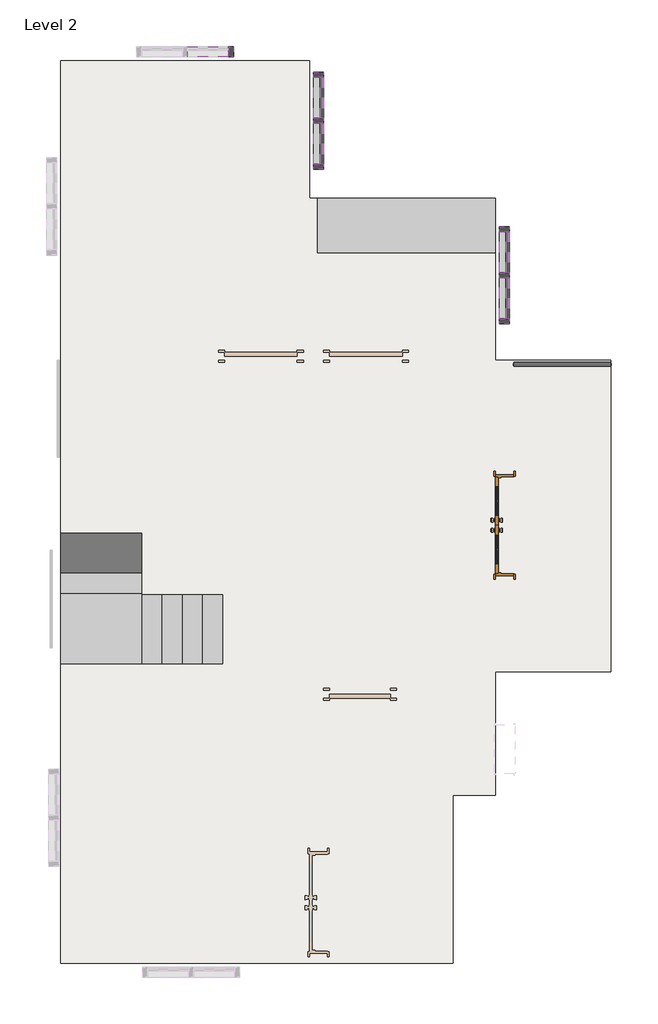
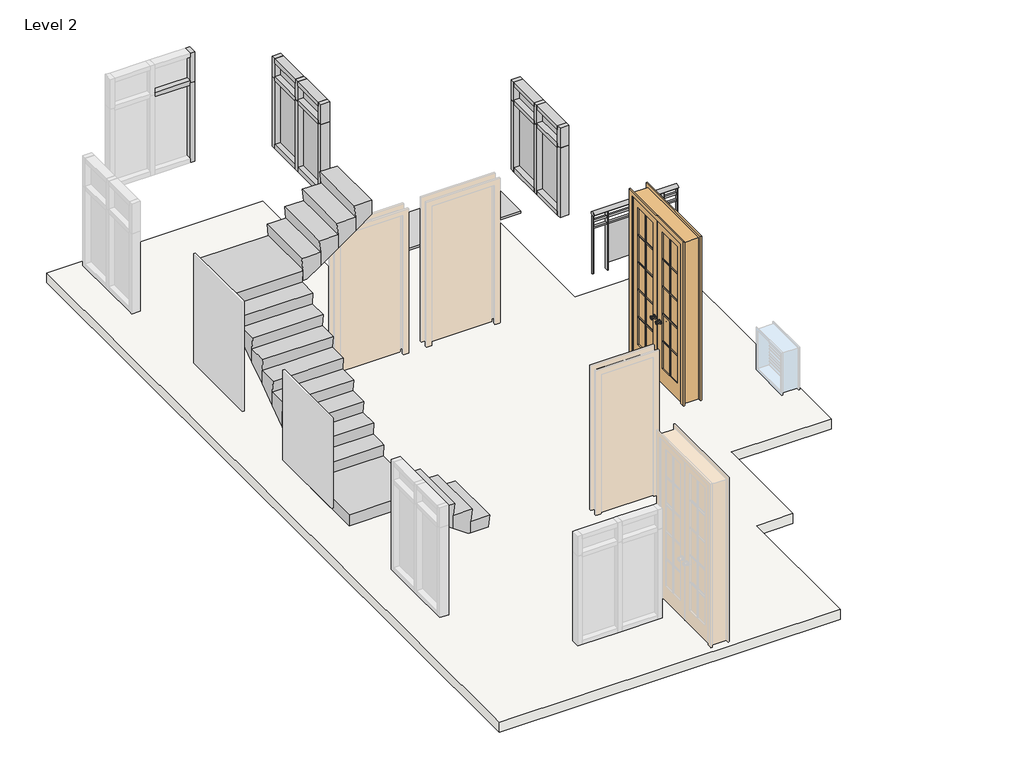
# One storey, part 2 of 2: 27 members, 8 plates, 1 door, 1 furniture element, 1 railing, 1 slab, 1 stair flight.
"""IFC4 building model written with IfcOpenShell, lengths in millimetres."""

from ifc_helpers import new_model, si_unit, point, frame, origin, place, context, project, spatial, polyline, ellipse_curve, trimmed, outline, extrude, faceted_brep, transform, mapped, element, save
from ifc_brep_helpers import plane_surface, extruded_surface, advanced_brep
from components import door_interior_double_full_glass_wood_4_x8_0c92ad92, casework_1_casework_1_edaa4522, member_0b7646a3, member_aaa03826, member_75074519, member_15823cb3, member_75d1e245, member_3c3dc66a, member_a715cb85, member_c4de40ee, system_panel_glazed_63160b6e, system_panel_glazed_4cc38c21

model = new_model("IFC4")

# Units and contexts
model_context = context("Model", 3, world=origin())
ifc_project = project(units=[si_unit("LENGTHUNIT", "METRE", prefix="MILLI")], contexts=[model_context])

# Site, building, storey
site = spatial("IfcSite", under=ifc_project)
building = spatial("IfcBuilding", under=site)
storey = spatial("IfcBuildingStorey", under=building, Name="Level 2", Elevation=609.6)

# Door
placement = place(None, origin())
door_interior_double_full_glass_wood_4_x8_shape = door_interior_double_full_glass_wood_4_x8_0c92ad92(model_context)
element("IfcDoor", 1, ObjectType="Door-Interior-Double-Full Glass-Wood : 4' x8'", at=placement, inside=storey, context=model_context, shape_type="MappedRepresentation", body=[
    mapped(door_interior_double_full_glass_wood_4_x8_shape, transform((738.4084347, 1540.0857557, 609.6), x_axis=(0.0, 1.0, 0.0), y_axis=(-1.0, 0.0, 0.0), z_axis=(0.0, 0.0, 1.0))),
])

# Furniture
casework_1_casework_1_shape = casework_1_casework_1_edaa4522(model_context)
element("IfcFurniture", 2, ObjectType="Casework 1 : Casework 1", at=placement, inside=storey, context=model_context, shape_type="MappedRepresentation", body=[
    mapped(casework_1_casework_1_shape, transform((0.0, 0.0, 0.0), x_axis=(1.0, 0.0, 0.0), y_axis=(0.0, 1.0, 0.0), z_axis=(0.0, 0.0, 1.0))),
])

# Members
member_shape = member_0b7646a3(model_context)
element("IfcMember", 3, ObjectType="Rectangular Mullion : 2.5\" x 5\" rectangular", at=placement, inside=storey, context=model_context, shape_type="MappedRepresentation", body=[
    mapped(member_shape, transform((-1595.2165653, 6068.4899592, 2895.6), x_axis=(0.0, 0.0, 1.0), y_axis=(-1.0, 0.0, 0.0), z_axis=(0.0, -1.0, 0.0))),
])
element("IfcMember", 4, ObjectType="Rectangular Mullion : 2.5\" x 5\" rectangular", at=placement, inside=storey, context=model_context, shape_type="MappedRepresentation", body=[
    mapped(member_shape, transform((-1595.2165653, 6646.3399592, 2895.6), x_axis=(0.0, 0.0, 1.0), y_axis=(-1.0, 0.0, 0.0), z_axis=(0.0, -1.0, 0.0))),
])
element("IfcMember", 5, ObjectType="Rectangular Mullion : 2.5\" x 5\" rectangular", at=placement, inside=storey, context=model_context, shape_type="MappedRepresentation", body=[
    mapped(member_shape, transform((741.5834347, 4130.8857559, 2895.6), x_axis=(0.0, 0.0, 1.0), y_axis=(-1.0, 0.0, 0.0), z_axis=(0.0, -1.0, 0.0))),
])
element("IfcMember", 6, ObjectType="Rectangular Mullion : 2.5\" x 5\" rectangular", at=placement, inside=storey, context=model_context, shape_type="MappedRepresentation", body=[
    mapped(member_shape, transform((741.5834347, 4708.7357559, 2895.6), x_axis=(0.0, 0.0, 1.0), y_axis=(-1.0, 0.0, 0.0), z_axis=(0.0, -1.0, 0.0))),
])
element("IfcMember", 7, ObjectType="Rectangular Mullion : 2.5\" x 5\" rectangular", at=placement, inside=storey, context=model_context, shape_type="MappedRepresentation", body=[
    mapped(member_shape, transform((-1595.2165653, 7160.6899592, 1524.0), x_axis=(0.0, 0.0, -1.0), y_axis=(-1.0, 0.0, 0.0), z_axis=(0.0, 1.0, 0.0))),
])
element("IfcMember", 8, ObjectType="Rectangular Mullion : 2.5\" x 5\" rectangular", at=placement, inside=storey, context=model_context, shape_type="MappedRepresentation", body=[
    mapped(member_shape, transform((-1595.2165653, 6582.8399592, 1524.0), x_axis=(0.0, 0.0, -1.0), y_axis=(-1.0, 0.0, 0.0), z_axis=(0.0, 1.0, 0.0))),
])
element("IfcMember", 9, ObjectType="Rectangular Mullion : 2.5\" x 5\" rectangular", at=placement, inside=storey, context=model_context, shape_type="MappedRepresentation", body=[
    mapped(member_shape, transform((741.5834347, 5223.0857559, 1524.0), x_axis=(0.0, 0.0, -1.0), y_axis=(-1.0, 0.0, 0.0), z_axis=(0.0, 1.0, 0.0))),
])
element("IfcMember", 10, ObjectType="Rectangular Mullion : 2.5\" x 5\" rectangular", at=placement, inside=storey, context=model_context, shape_type="MappedRepresentation", body=[
    mapped(member_shape, transform((741.5834347, 4645.2357559, 1524.0), x_axis=(0.0, 0.0, -1.0), y_axis=(-1.0, 0.0, 0.0), z_axis=(0.0, 1.0, 0.0))),
])
member_2_shape = member_aaa03826(model_context)
element("IfcMember", 11, ObjectType="Rectangular Mullion : 2.5\" x 5\" rectangular", at=placement, inside=storey, context=model_context, shape_type="MappedRepresentation", body=[
    mapped(member_2_shape, transform((-2725.5165655, 7483.6857557, 2743.2), x_axis=(0.0, 0.0, 1.0), y_axis=(0.0, -1.0, 0.0), z_axis=(1.0, 0.0, 0.0))),
])
element("IfcMember", 12, ObjectType="Rectangular Mullion : 2.5\" x 5\" rectangular", at=placement, inside=storey, context=model_context, shape_type="MappedRepresentation", body=[
    mapped(member_2_shape, transform((-1595.2165653, 6646.3399592, 2590.8), x_axis=(0.0, 0.0, 1.0), y_axis=(-1.0, 0.0, 0.0), z_axis=(0.0, -1.0, 0.0))),
])
element("IfcMember", 13, ObjectType="Rectangular Mullion : 2.5\" x 5\" rectangular", at=placement, inside=storey, context=model_context, shape_type="MappedRepresentation", body=[
    mapped(member_2_shape, transform((-1595.2165653, 6068.4899592, 2590.8), x_axis=(0.0, 0.0, 1.0), y_axis=(-1.0, 0.0, 0.0), z_axis=(0.0, -1.0, 0.0))),
])
element("IfcMember", 14, ObjectType="Rectangular Mullion : 2.5\" x 5\" rectangular", at=placement, inside=storey, context=model_context, shape_type="MappedRepresentation", body=[
    mapped(member_2_shape, transform((741.5834347, 4708.7357559, 2590.8), x_axis=(0.0, 0.0, 1.0), y_axis=(-1.0, 0.0, 0.0), z_axis=(0.0, -1.0, 0.0))),
])
element("IfcMember", 15, ObjectType="Rectangular Mullion : 2.5\" x 5\" rectangular", at=placement, inside=storey, context=model_context, shape_type="MappedRepresentation", body=[
    mapped(member_2_shape, transform((741.5834347, 4130.8857559, 2590.8), x_axis=(0.0, 0.0, 1.0), y_axis=(-1.0, 0.0, 0.0), z_axis=(0.0, -1.0, 0.0))),
])
member_3_shape = member_75074519(model_context)
element("IfcMember", 16, ObjectType="Rectangular Mullion : 2.5\" x 5\" rectangular", at=placement, inside=storey, context=model_context, shape_type="MappedRepresentation", body=[
    mapped(member_3_shape, transform((-2662.0165655, 7483.6857557, 1524.0), x_axis=(1.0, 0.0, 0.0), y_axis=(0.0, -1.0, 0.0), z_axis=(0.0, 0.0, -1.0))),
])
member_4_shape = member_15823cb3(model_context)
element("IfcMember", 17, ObjectType="Rectangular Mullion : 2.5\" x 5\" rectangular", at=placement, inside=storey, context=model_context, shape_type="MappedRepresentation", body=[
    mapped(member_4_shape, transform((-2662.0165655, 7483.6857557, 2743.2), x_axis=(1.0, 0.0, 0.0), y_axis=(0.0, -1.0, 0.0), z_axis=(0.0, 0.0, -1.0))),
])
member_5_shape = member_75d1e245(model_context)
element("IfcMember", 18, ObjectType="Rectangular Mullion : 2.5\" x 5\" rectangular", at=placement, inside=storey, context=model_context, shape_type="MappedRepresentation", body=[
    mapped(member_5_shape, transform((-1595.2165653, 6614.5899592, 2590.8), x_axis=(0.0, -1.0, 0.0), y_axis=(-1.0, 0.0, 0.0), z_axis=(0.0, 0.0, -1.0))),
])
element("IfcMember", 19, ObjectType="Rectangular Mullion : 2.5\" x 5\" rectangular", at=placement, inside=storey, context=model_context, shape_type="MappedRepresentation", body=[
    mapped(member_5_shape, transform((741.5834347, 4676.9857559, 2590.8), x_axis=(0.0, -1.0, 0.0), y_axis=(-1.0, 0.0, 0.0), z_axis=(0.0, 0.0, -1.0))),
])
member_6_shape = member_3c3dc66a(model_context)
element("IfcMember", 20, ObjectType="Rectangular Mullion : 2.5\" x 5\" rectangular", at=placement, inside=storey, context=model_context, shape_type="MappedRepresentation", body=[
    mapped(member_6_shape, transform((-1595.2165653, 7224.1899592, 2895.6), x_axis=(0.0, 1.0, 0.0), y_axis=(-1.0, 0.0, 0.0), z_axis=(0.0, 0.0, 1.0))),
])
element("IfcMember", 21, ObjectType="Rectangular Mullion : 2.5\" x 5\" rectangular", at=placement, inside=storey, context=model_context, shape_type="MappedRepresentation", body=[
    mapped(member_6_shape, transform((741.5834347, 5286.5857559, 2895.6), x_axis=(0.0, 1.0, 0.0), y_axis=(-1.0, 0.0, 0.0), z_axis=(0.0, 0.0, 1.0))),
])
element("IfcMember", 22, ObjectType="Rectangular Mullion : 2.5\" x 5\" rectangular", at=placement, inside=storey, context=model_context, shape_type="MappedRepresentation", body=[
    mapped(member_6_shape, transform((-1595.2165653, 6004.9899592, 2590.8), x_axis=(0.0, -1.0, 0.0), y_axis=(-1.0, 0.0, 0.0), z_axis=(0.0, 0.0, -1.0))),
])
element("IfcMember", 23, ObjectType="Rectangular Mullion : 2.5\" x 5\" rectangular", at=placement, inside=storey, context=model_context, shape_type="MappedRepresentation", body=[
    mapped(member_6_shape, transform((741.5834347, 4067.3857559, 2590.8), x_axis=(0.0, -1.0, 0.0), y_axis=(-1.0, 0.0, 0.0), z_axis=(0.0, 0.0, -1.0))),
])
member_7_shape = member_a715cb85(model_context)
element("IfcMember", 24, ObjectType="Rectangular Mullion : 2.5\" x 5\" rectangular", at=placement, inside=storey, context=model_context, shape_type="MappedRepresentation", body=[
    mapped(member_7_shape, transform((-1595.2165653, 6614.5899592, 1524.0), x_axis=(0.0, -1.0, 0.0), y_axis=(-1.0, 0.0, 0.0), z_axis=(0.0, 0.0, -1.0))),
])
element("IfcMember", 25, ObjectType="Rectangular Mullion : 2.5\" x 5\" rectangular", at=placement, inside=storey, context=model_context, shape_type="MappedRepresentation", body=[
    mapped(member_7_shape, transform((741.5834347, 4676.9857559, 1524.0), x_axis=(0.0, -1.0, 0.0), y_axis=(-1.0, 0.0, 0.0), z_axis=(0.0, 0.0, -1.0))),
])
member_8_shape = member_c4de40ee(model_context)
element("IfcMember", 26, ObjectType="Rectangular Mullion : 2.5\" x 5\" rectangular", at=placement, inside=storey, context=model_context, shape_type="MappedRepresentation", body=[
    mapped(member_8_shape, transform((-1595.2165653, 6004.9899592, 1524.0), x_axis=(0.0, -1.0, 0.0), y_axis=(-1.0, 0.0, 0.0), z_axis=(0.0, 0.0, -1.0))),
])
element("IfcMember", 27, ObjectType="Rectangular Mullion : 2.5\" x 5\" rectangular", at=placement, inside=storey, context=model_context, shape_type="MappedRepresentation", body=[
    mapped(member_8_shape, transform((741.5834347, 4067.3857559, 1524.0), x_axis=(0.0, -1.0, 0.0), y_axis=(-1.0, 0.0, 0.0), z_axis=(0.0, 0.0, -1.0))),
])
element("IfcMember", 28, ObjectType="Rectangular Mullion : 2.5\" x 5\" rectangular", at=placement, inside=storey, context=model_context, shape_type="MappedRepresentation", body=[
    mapped(member_8_shape, transform((-1595.2165653, 7224.1899592, 2590.8), x_axis=(0.0, 1.0, 0.0), y_axis=(-1.0, 0.0, 0.0), z_axis=(0.0, 0.0, 1.0))),
])
element("IfcMember", 29, ObjectType="Rectangular Mullion : 2.5\" x 5\" rectangular", at=placement, inside=storey, context=model_context, shape_type="MappedRepresentation", body=[
    mapped(member_8_shape, transform((741.5834347, 5286.5857559, 2590.8), x_axis=(0.0, 1.0, 0.0), y_axis=(-1.0, 0.0, 0.0), z_axis=(0.0, 0.0, 1.0))),
])

# Plates
system_panel_glazed_shape = system_panel_glazed_63160b6e(model_context)
element("IfcPlate", 30, ObjectType="System Panel : Glazed", at=placement, inside=storey, context=model_context, shape_type="MappedRepresentation", body=[
    mapped(system_panel_glazed_shape, transform((741.5834347, 4965.9107559, 2622.55), x_axis=(0.0, -1.0, 0.0), y_axis=(1.0, 0.0, 0.0), z_axis=(0.0, 0.0, 1.0))),
])
element("IfcPlate", 31, ObjectType="System Panel : Glazed", at=placement, inside=storey, context=model_context, shape_type="MappedRepresentation", body=[
    mapped(system_panel_glazed_shape, transform((741.5834347, 4388.0607559, 2622.55), x_axis=(0.0, -1.0, 0.0), y_axis=(1.0, 0.0, 0.0), z_axis=(0.0, 0.0, 1.0))),
])
element("IfcPlate", 32, ObjectType="System Panel : Glazed", at=placement, inside=storey, context=model_context, shape_type="MappedRepresentation", body=[
    mapped(system_panel_glazed_shape, transform((-1595.2165653, 6903.5149592, 2622.55), x_axis=(0.0, -1.0, 0.0), y_axis=(1.0, 0.0, 0.0), z_axis=(0.0, 0.0, 1.0))),
])
element("IfcPlate", 33, ObjectType="System Panel : Glazed", at=placement, inside=storey, context=model_context, shape_type="MappedRepresentation", body=[
    mapped(system_panel_glazed_shape, transform((-1595.2165653, 6325.6649592, 2622.55), x_axis=(0.0, -1.0, 0.0), y_axis=(1.0, 0.0, 0.0), z_axis=(0.0, 0.0, 1.0))),
])
system_panel_glazed_2_shape = system_panel_glazed_4cc38c21(model_context)
element("IfcPlate", 34, ObjectType="System Panel : Glazed", at=placement, inside=storey, context=model_context, shape_type="MappedRepresentation", body=[
    mapped(system_panel_glazed_2_shape, transform((-1595.2165653, 6903.5149592, 1587.5), x_axis=(0.0, -1.0, 0.0), y_axis=(1.0, 0.0, 0.0), z_axis=(0.0, 0.0, 1.0))),
])
element("IfcPlate", 35, ObjectType="System Panel : Glazed", at=placement, inside=storey, context=model_context, shape_type="MappedRepresentation", body=[
    mapped(system_panel_glazed_2_shape, transform((741.5834347, 4965.9107559, 1587.5), x_axis=(0.0, -1.0, 0.0), y_axis=(1.0, 0.0, 0.0), z_axis=(0.0, 0.0, 1.0))),
])
element("IfcPlate", 36, ObjectType="System Panel : Glazed", at=placement, inside=storey, context=model_context, shape_type="MappedRepresentation", body=[
    mapped(system_panel_glazed_2_shape, transform((741.5834347, 4388.0607559, 1587.5), x_axis=(0.0, -1.0, 0.0), y_axis=(1.0, 0.0, 0.0), z_axis=(0.0, 0.0, 1.0))),
])
element("IfcPlate", 37, ObjectType="System Panel : Glazed", at=placement, inside=storey, context=model_context, shape_type="MappedRepresentation", body=[
    mapped(system_panel_glazed_2_shape, transform((-1595.2165653, 6325.6649592, 1587.5), x_axis=(0.0, -1.0, 0.0), y_axis=(1.0, 0.0, 0.0), z_axis=(0.0, 0.0, 1.0))),
])

# Railing
element("IfcRailing", 38, ObjectType="Glass Panel - Bottom Fill", at=placement, inside=storey, context=model_context, shape_type="SolidModel", body=[
    advanced_brep(
    [(855.8834347, 3597.4857557, 1828.8), (855.8834347, 3521.2857557, 1828.8), (2075.0834347, 3597.4857557, 1828.8), (2075.0834347, 3521.2857557, 1828.8)],
    [
        (0, 1, ellipse_curve(frame((855.8834347, 3559.3857557, 1828.8), z_axis=(-1.0, 0.0, 0.0), x_axis=(0.0, -1.0, 0.0)), 38.1, 28.575)),
        (1, 0, ellipse_curve(frame((855.8834347, 3559.3857557, 1828.8), z_axis=(-1.0, 0.0, 0.0), x_axis=(0.0, -1.0, 0.0)), 38.1, 28.575)),
        (2, 3, ellipse_curve(frame((2075.0834347, 3559.3857557, 1828.8), z_axis=(1.0, 0.0, 0.0), x_axis=(0.0, -1.0, 0.0)), 38.1, 28.575)),
        (3, 2, ellipse_curve(frame((2075.0834347, 3559.3857557, 1828.8), z_axis=(1.0, 0.0, 0.0), x_axis=(0.0, -1.0, 0.0)), 38.1, 28.575)),
        (0, 2),
        (3, 1),
    ],
    [
        plane_surface(frame((855.8834347, 3559.3857557, 1828.8), z_axis=(-1.0, 0.0, 0.0), x_axis=(0.0, 1.0, 0.0))),
        plane_surface(frame((2075.0834347, 3559.3857557, 1828.8), z_axis=(1.0, 0.0, 0.0), x_axis=(0.0, 1.0, 0.0))),
        extruded_surface(trimmed(ellipse_curve(frame((2075.0834347, 3559.3857557, 1828.8), z_axis=(-1.0, 0.0, 0.0), x_axis=(0.0, -1.0, 0.0)), 38.1, 28.575), [point((2075.0834347, 3597.4857557, 1828.8))], [point((2075.0834347, 3521.2857557, 1828.8))], True, "CARTESIAN"), (-1219.2, 0.0, 0.0), 1219.2),
        extruded_surface(trimmed(ellipse_curve(frame((2075.0834347, 3559.3857557, 1828.8), z_axis=(-1.0, 0.0, 0.0), x_axis=(0.0, -1.0, 0.0)), 38.1, 28.575), [point((2075.0834347, 3521.2857557, 1828.8))], [point((2075.0834347, 3597.4857557, 1828.8))], True, "CARTESIAN"), (-1219.2, 0.0, 0.0), 1219.2),
    ],
    [
        (0, [[1, 2]]),
        (1, [[3, 4]]),
        (2, [[-1, 5, -4, 6]]),
        (3, [[-2, -6, -3, -5]]),
    ],
),
    extrude(outline(polyline([(855.8834347, 3546.6857557), (855.8834347, 3572.0857557), (2075.0834347, 3572.0857557), (2075.0834347, 3546.6857557), (855.8834347, 3546.6857557)])), frame((0.0, 0.0, 1714.5), z_axis=(0.0, 0.0, 1.0), x_axis=(1.0, 0.0, 0.0)), (0.0, 0.0, 1.0), 25.4),
    extrude(outline(polyline([(855.8834347, 3546.6857557), (855.8834347, 3572.0857557), (2075.0834347, 3572.0857557), (2075.0834347, 3546.6857557), (855.8834347, 3546.6857557)])), frame((0.0, 0.0, 1612.9), z_axis=(0.0, 0.0, 1.0), x_axis=(1.0, 0.0, 0.0)), (0.0, 0.0, 1.0), 25.4),
    extrude(outline(polyline([(1865.5334347, 3533.9857557), (1865.5334347, 3584.7857557), (1878.2334347, 3584.7857557), (1878.2334347, 3533.9857557), (1865.5334347, 3533.9857557)])), frame((0.0, 0.0, 914.4), z_axis=(0.0, 0.0, 1.0), x_axis=(1.0, 0.0, 0.0)), (0.0, 0.0, 1.0), 885.825),
    extrude(outline(polyline([(1059.0834347, 3565.9209127), (1871.8834347, 3565.9209127), (1871.8834347, 3559.5709127), (1059.0834347, 3559.5709127), (1059.0834347, 3565.9209127)])), frame((0.0, 0.0, 1016.0), z_axis=(0.0, 0.0, 1.0), x_axis=(1.0, 0.0, 0.0)), (0.0, 0.0, 1.0), 596.9),
    extrude(outline(polyline([(1052.7334347, 3533.9857557), (1052.7334347, 3584.7857557), (1065.4334347, 3584.7857557), (1065.4334347, 3533.9857557), (1052.7334347, 3533.9857557)])), frame((0.0, 0.0, 914.4), z_axis=(0.0, 0.0, 1.0), x_axis=(1.0, 0.0, 0.0)), (0.0, 0.0, 1.0), 885.825),
    extrude(outline(polyline([(2062.3834347, 3549.8607557), (2062.3834347, 3568.9107557), (2081.4334347, 3568.9107557), (2081.4334347, 3549.8607557), (2062.3834347, 3549.8607557)])), frame((0.0, 0.0, 914.4), z_axis=(0.0, 0.0, 1.0), x_axis=(1.0, 0.0, 0.0)), (0.0, 0.0, 1.0), 885.825),
    extrude(outline(polyline([(849.5334347, 3549.8607557), (849.5334347, 3568.9107557), (868.5834347, 3568.9107557), (868.5834347, 3549.8607557), (849.5334347, 3549.8607557)])), frame((0.0, 0.0, 914.4), z_axis=(0.0, 0.0, 1.0), x_axis=(1.0, 0.0, 0.0)), (0.0, 0.0, 1.0), 885.825),
])

# Slab
element("IfcSlab", 39, ObjectType="6\" floor", at=placement, inside=storey, context=model_context, shape_type="SweptSolid", body=[
    extrude(outline(polyline([(-1709.5165653, 7369.3857557), (-1709.5165653, 5642.1857557), (627.2834347, 5642.1857557), (627.2834347, 3610.1857557), (2075.0834347, 3610.1857557), (2075.0834347, -301.4142443), (627.2834347, -301.4142443), (627.2834347, -1850.8142443), (93.8834347, -1850.8142443), (93.8834347, -3959.0142443), (-4833.7165653, -3959.0142443), (-4833.7165653, 7369.3857557), (-1709.5165653, 7369.3857557)])), frame((0.0, 0.0, 457.2), z_axis=(0.0, 0.0, 1.0), x_axis=(1.0, 0.0, 0.0)), (0.0, 0.0, 1.0), 152.4),
])

# Stair flight
element("IfcStairFlight", 40, ObjectType="3/4\" Nosing 6 1/2\" Depth", at=placement, inside=storey, context=model_context, shape_type="Brep", body=[
    faceted_brep([(-2801.7165653, 663.7857557, 787.4), (-2801.7165653, -199.8142443, 787.4), (-2820.7665653, -199.8142443, 609.6), (-2820.7665653, 663.7857557, 609.6), (-3074.7665653, 663.7857557, 787.4), (-3074.7665653, -199.8142443, 787.4), (-3074.7665653, -199.8142443, 609.6), (-3074.7665653, 663.7857557, 609.6), (-3055.7165653, -199.8142443, 965.2), (-3055.7165653, 663.7857557, 965.2), (-3328.7665653, 663.7857557, 965.2), (-3328.7665653, -199.8142443, 965.2), (-3328.7665653, -199.8142443, 763.6697668), (-3108.6668985, -199.8142443, 609.6), (-3108.6668985, 663.7857557, 609.6), (-3328.7665653, 663.7857557, 763.6697668), (-3309.7165653, -199.8142443, 1143.0), (-3309.7165653, 663.7857557, 1143.0), (-3582.7665653, 663.7857557, 1143.0), (-3582.7665653, -199.8142443, 1143.0), (-3582.7665653, -199.8142443, 941.4697668), (-3582.7665653, 663.7857557, 941.4697668), (-3563.7165653, -199.8142443, 1320.8), (-3563.7165653, 663.7857557, 1320.8), (-3836.7665653, 663.7857557, 1320.8), (-3836.7665653, -199.8142443, 1320.8), (-3836.7665653, -199.8142443, 1119.2697668), (-4142.8097556, 663.7857557, 1333.5), (-3835.405851, 663.7857557, 1333.5), (-4833.7165653, 704.6678432, 1498.6), (-4833.7165653, -199.8142443, 1498.6), (-4142.8097556, -199.8142443, 1498.6), (-3817.7165653, -199.8142443, 1498.6), (-3817.7165653, 663.7857557, 1498.6), (-3817.7165653, 704.6678432, 1498.6), (-4833.7165653, 704.6678432, 1333.5), (-4833.7165653, -199.8142443, 1333.5), (-4142.8097556, -199.8142443, 1333.5), (-3817.7165653, 663.7857557, 1333.5), (-3817.7165653, 704.6678432, 1333.5), (-4833.7165653, 685.6178432, 1676.4), (-3817.7165653, 685.6178432, 1676.4), (-3817.7165653, 756.7110335, 1676.4), (-3817.7165653, 958.6678432, 1676.4), (-4833.7165653, 958.6678432, 1676.4), (-4833.7165653, 756.7110335, 1676.4), (-4833.7165653, 958.6678432, 1474.8697668), (-4833.7165653, 756.7110335, 1333.5), (-3817.7165653, 756.7110335, 1333.5), (-3817.7165653, 958.6678432, 1474.8697668), (-4833.7165653, 939.6178432, 1854.2), (-3817.7165653, 939.6178432, 1854.2), (-3817.7165653, 1212.6678432, 1854.2), (-4833.7165653, 1212.6678432, 1854.2), (-4833.7165653, 1212.6678432, 1652.6697668), (-3817.7165653, 1212.6678432, 1652.6697668), (-4833.7165653, 1193.6178432, 2032.0), (-3817.7165653, 1193.6178432, 2032.0), (-3817.7165653, 1466.6678432, 2032.0), (-4833.7165653, 1466.6678432, 2032.0), (-4833.7165653, 1466.6678432, 1830.4697668), (-3817.7165653, 1466.6678432, 1830.4697668), (-4833.7165653, 1447.6178432, 2209.8), (-3817.7165653, 1447.6178432, 2209.8), (-3817.7165653, 1720.6678432, 2209.8), (-4833.7165653, 1720.6678432, 2209.8), (-4833.7165653, 1720.6678432, 2008.2697668), (-3817.7165653, 1720.6678432, 2008.2697668), (-4833.7165653, 1701.6178432, 2387.6), (-3817.7165653, 1701.6178432, 2387.6), (-3817.7165653, 1974.6678432, 2387.6), (-4833.7165653, 1974.6678432, 2387.6), (-4833.7165653, 1974.6678432, 2186.0697668), (-3817.7165653, 1974.6678432, 2186.0697668), (-4833.7165653, 1955.6178432, 2565.4), (-3817.7165653, 1955.6178432, 2565.4), (-3817.7165653, 2228.6678432, 2565.4), (-4833.7165653, 2228.6678432, 2565.4), (-4833.7165653, 2228.6678432, 2363.8697668), (-3817.7165653, 2228.6678432, 2363.8697668), (-4833.7165653, 2209.6178432, 2743.2), (-3817.7165653, 2209.6178432, 2743.2), (-3817.7165653, 2482.6678432, 2743.2), (-4833.7165653, 2482.6678432, 2743.2), (-4833.7165653, 2482.6678432, 2541.6697668), (-3817.7165653, 2482.6678432, 2541.6697668), (-4833.7165653, 2463.6178432, 2921.0), (-3817.7165653, 2463.6178432, 2921.0), (-3817.7165653, 2736.6678432, 2921.0), (-4833.7165653, 2736.6678432, 2921.0), (-4833.7165653, 2736.6678432, 2719.4697668), (-3817.7165653, 2736.6678432, 2719.4697668), (-3798.6665653, 3610.1857557, 3098.8), (-4833.7165653, 3610.1857557, 3098.8), (-4833.7165653, 3042.7110335, 3098.8), (-4833.7165653, 2717.6178432, 3098.8), (-3817.7165653, 2717.6178432, 3098.8), (-3817.7165653, 2746.5857557, 3098.8), (-3798.6665653, 2746.5857557, 3098.8), (-3798.6665653, 3610.1857557, 2933.7), (-4833.7165653, 3610.1857557, 2933.7), (-4833.7165653, 3042.7110335, 2933.7), (-3817.7165653, 3042.7110335, 2933.7), (-3817.7165653, 2746.5857557, 2933.7), (-3798.6665653, 2746.5857557, 2933.7), (-3817.7165653, 3610.1857557, 3276.6), (-3817.7165653, 2746.5857557, 3276.6), (-3746.623375, 2746.5857557, 3276.6), (-3544.6665653, 2746.5857557, 3276.6), (-3544.6665653, 3610.1857557, 3276.6), (-3746.623375, 3610.1857557, 3276.6), (-3544.6665653, 3610.1857557, 3075.0697668), (-3746.623375, 3610.1857557, 2933.7), (-3746.623375, 2746.5857557, 2933.7), (-3544.6665653, 2746.5857557, 3075.0697668), (-3563.7165653, 3610.1857557, 3454.4), (-3563.7165653, 2746.5857557, 3454.4), (-3290.6665653, 2746.5857557, 3454.4), (-3290.6665653, 3610.1857557, 3454.4), (-3290.6665653, 3610.1857557, 3252.8697668), (-3290.6665653, 2746.5857557, 3252.8697668), (-3309.7165653, 3610.1857557, 3632.2), (-3309.7165653, 2746.5857557, 3632.2), (-3036.6665653, 2746.5857557, 3632.2), (-3036.6665653, 3610.1857557, 3632.2), (-3036.6665653, 3610.1857557, 3430.6697668), (-3036.6665653, 2746.5857557, 3430.6697668), (-3055.7165653, 3610.1857557, 3810.0), (-3055.7165653, 2746.5857557, 3810.0), (-2801.7165653, 2746.5857557, 3810.0), (-2801.7165653, 3610.1857557, 3810.0), (-2801.7165653, 3610.1857557, 3595.1347668), (-2801.7165653, 2746.5857557, 3595.1347668)], [[[0, 1, 2, 3]], [[1, 0, 4, 5]], [[1, 5, 6, 2]], [[4, 0, 3, 7]], [[8, 9, 10, 11]], [[6, 5, 8, 11, 12, 13]], [[4, 7, 14, 15, 10, 9]], [[5, 4, 9, 8]], [[16, 17, 18, 19]], [[16, 19, 20, 12, 11]], [[18, 17, 10, 15, 21]], [[11, 10, 17, 16]], [[22, 23, 24, 25]], [[22, 25, 26, 20, 19]], [[23, 18, 21, 27, 28, 24]], [[19, 18, 23, 22]], [[29, 30, 31, 32, 33, 34]], [[30, 29, 35, 36]], [[25, 32, 31, 30, 36, 37, 26]], [[33, 28, 38]], [[34, 33, 38, 39]], [[25, 24, 28, 33, 32]], [[40, 41, 42, 43, 44, 45]], [[29, 40, 45, 44, 46, 47, 35]], [[41, 34, 39, 48, 49, 43, 42]], [[29, 34, 41, 40]], [[50, 51, 52, 53]], [[50, 53, 54, 46, 44]], [[52, 51, 43, 49, 55]], [[44, 43, 51, 50]], [[56, 57, 58, 59]], [[56, 59, 60, 54, 53]], [[58, 57, 52, 55, 61]], [[53, 52, 57, 56]], [[62, 63, 64, 65]], [[62, 65, 66, 60, 59]], [[64, 63, 58, 61, 67]], [[59, 58, 63, 62]], [[68, 69, 70, 71]], [[68, 71, 72, 66, 65]], [[70, 69, 64, 67, 73]], [[65, 64, 69, 68]], [[74, 75, 76, 77]], [[74, 77, 78, 72, 71]], [[76, 75, 70, 73, 79]], [[71, 70, 75, 74]], [[80, 81, 82, 83]], [[80, 83, 84, 78, 77]], [[82, 81, 76, 79, 85]], [[77, 76, 81, 80]], [[86, 87, 88, 89]], [[86, 89, 90, 84, 83]], [[88, 87, 82, 85, 91]], [[83, 82, 87, 86]], [[92, 93, 94, 95, 96, 97, 98]], [[93, 92, 99, 100]], [[89, 95, 94, 93, 100, 101, 90]], [[97, 96, 88, 91, 102, 103]], [[98, 97, 103, 104]], [[89, 88, 96, 95]], [[105, 106, 107, 108, 109, 110]], [[92, 105, 110, 109, 111, 112, 99]], [[106, 98, 104, 113, 114, 108, 107]], [[92, 98, 106, 105]], [[115, 116, 117, 118]], [[115, 118, 119, 111, 109]], [[117, 116, 108, 114, 120]], [[109, 108, 116, 115]], [[121, 122, 123, 124]], [[121, 124, 125, 119, 118]], [[123, 122, 117, 120, 126]], [[118, 117, 122, 121]], [[127, 128, 129, 130]], [[127, 130, 131, 125, 124]], [[129, 128, 123, 126, 132]], [[130, 129, 132, 131]], [[124, 123, 128, 127]], [[2, 6, 13, 14, 7, 3]], [[37, 27, 21, 15, 14, 13, 12, 20, 26]], [[27, 37, 36, 35, 47, 48, 39, 38, 28]], [[48, 47, 46, 54, 60, 66, 72, 78, 84, 90, 101, 102, 91, 85, 79, 73, 67, 61, 55, 49]], [[102, 101, 100, 99, 112, 113, 104, 103]], [[113, 112, 111, 119, 125, 131, 132, 126, 120, 114]]]),
])

save(model, "model.ifc")

# Revit data of these elements
# Type "Door-Interior-Double-Full Glass-Wood : 4' x8'"
#   Type Mark = "14"
#   Assembly Code = "C1020300"
#   Analytic Construction = "French door, wood frame with single glass"
#   Top Rail = 0' - 4 11/16"
#   Thickness = 0' - 1 3/8"
#   Thermal Resistance (R) = 1.0696 (h·ft²·°F)/BTU
#   Swing Angle [instance default] = 90.00°
#   Stiles = 0' - 4 3/4"
#   Rough Width = 4' - 2"
#   Rough Height = 8' - 1"
#   Panel Width = 2' - 0"
#   Height = 8' - 0"
#   Width = 4' - 0"
#   Heat Transfer Coefficient (U) = 0.9350 BTU/(h·ft²·°F)
#   Bottom Rail = 0' - 9 1/8"
#   Show Grill [instance default] = yes
#   Trim Material = Cherry
#   Panel Material = Cherry
#   Frame Material = Cherry
#   Door Handle Material = Aluminum
#   Visual Light Transmittance = 0
#   Solar Heat Gain Coefficient = 0
#   Wall Closure = (empty or 0)
#   Function = (empty or 0)
# Type "Rectangular Mullion : 2.5\" x 5\" rectangular"
#   built-in parameter 1007304 = 0.416667 (stored number, unit not read)
#   built-in parameter 1007301 = 0.104167 (stored number, unit not read)
#   built-in parameter 1007300 = 0.104167 (stored number, unit not read)
# Type "System Panel : Glazed"
#   Construction Type Id = "GSP4R"
#   Analytic Construction = "1/8 in Pilkington single glazing"
#   Visual Light Transmittance = 0.9
#   Solar Heat Gain Coefficient = 0.86
#   Heat Transfer Coefficient (U) = 1.18115 BTU/(h·ft²·°F)
#   Define Thermal Properties by = 1
# Type "Glass Panel - Bottom Fill"
#   Assembly Code = "C2010400"
#   built-in parameter 1008612 = 0.0416667 (stored number, unit not read)
#   built-in parameter 1008611 = 0.0416667 (stored number, unit not read)
#   built-in parameter 1008609 = 0.333333 (stored number, unit not read)
#   built-in parameter 1008604 = 0.166667 (stored number, unit not read)
#   built-in parameter 1008603 = 0.166667 (stored number, unit not read)
#   Railing Height = 3' - 0"
#   built-in parameter 1008630 = 2
#   built-in parameter 1008610 = 2
#   built-in parameter 1008618 = Baluster - Square : 3/4"
# Type "6\" floor"
#   Assembly Code = "B1010"
#   Function = 0
#   Layers, outside or top first: 0' - 6" no material (function 1)
# Element 1 (IfcDoor, "Door-Interior-Double-Full Glass-Wood : 4' x8'")
#   Swing Angle = 45.00°
#   Show Grill = yes
#   Phase Created = New Construction
#   Materials on its faces: "Cherry", "Aluminum", "Glass"
# Element 2 (IfcFurniture, "Casework 1 : Casework 1")
#   Phase Created = New Construction
# Elements 3, 4, 5, 6, 7, 8, 9, 10, 11, 12, 13, 14, 15, 16, 17, 18, 19, 20, 21, 22, 23, 24, 25, 26, 27, 28, 29 (IfcMember, "Rectangular Mullion : 2.5\" x 5\" rectangular")
#   Phase Created = New Construction
#   Materials on its faces: "Aluminum"
# Elements 30, 31, 32, 33, 34, 35, 36, 37 (IfcPlate, "System Panel : Glazed")
#   Phase Created = New Construction
#   Materials on its faces: "Glass"
# Element 38 (IfcRailing, "Glass Panel - Bottom Fill")
#   built-in parameter 1008621 = 1 (stored number, unit not read)
#   Phase Created = New Construction
#   Materials on its faces: "Glass"
# Element 39 (IfcSlab, "6\" floor")
#   Height Offset From Level = 0' - 0"
#   Phase Created = New Construction
#   Materials on its faces: "Default Floor"
# Element 40 (IfcStairFlight, "3/4\" Nosing 6 1/2\" Depth")
#   Phase Created = New Construction
#   Materials on its faces: "Concrete, Cast-in-Place gray"
# Materials
#   "Cherry": class "Wood", colour RGB 226 177 128, transparency 0, Description = "Prunus Serotina", Cost = 0
#   "Aluminum": class "Metal", colour RGB 247 247 247, transparency 0, Description = "Aluminum 6061", Cost = 0
#   "Glass": class "Glass", colour RGB 0 128 192, transparency 0.75, Description = "Soda Lime Glass", Cost = 0
#   "Default Floor": colour RGB 128 128 128, transparency 0, Cost = 0
#   "Concrete, Cast-in-Place gray": class "Concrete", colour RGB 192 192 192, transparency 0, Description = "Cast-in-place concrete", Cost = 0
